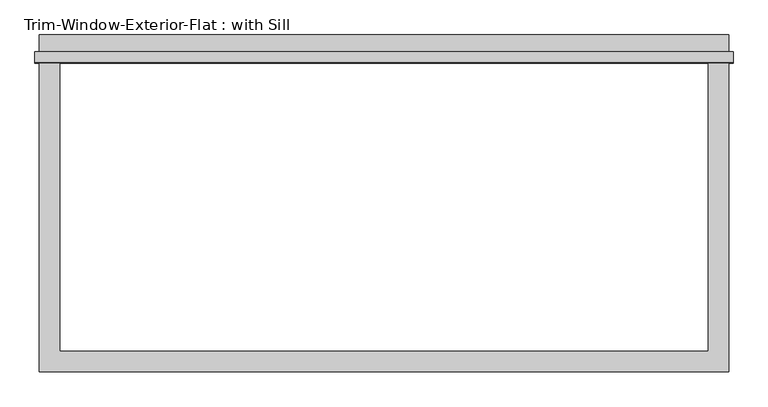
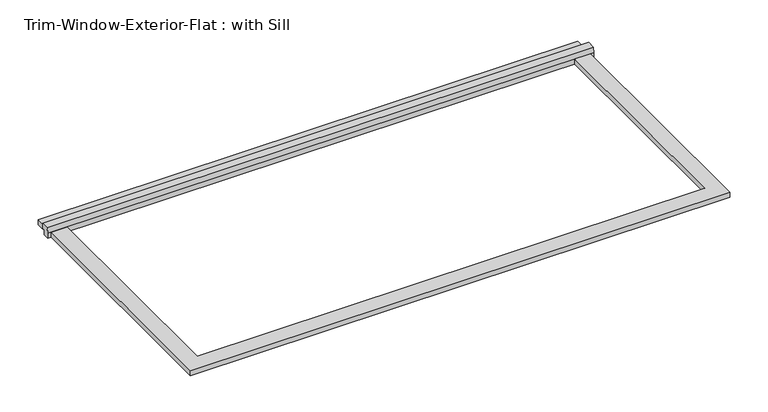
"""IFC4 building model written with IfcOpenShell, lengths in millimetres: proxy geometry, Trim-Window-Exterior-Flat : with Sill."""

from ifc_helpers import new_model, si_unit, frame, origin, origin_with_axes, place, context, project, spatial, polyline, outline, extrude, source, transform, mapped, element, save


def trim_window_exterior_flat_with_sill_7b949e88(model_context):
    return source(origin(), model_context, "Body", "SweptSolid", [
        extrude(outline(polyline([(971.55, 834.9823709), (-971.55, 834.9823709), (-971.55, 892.1323709), (971.55, 892.1323709), (971.55, 834.9823709)])), origin_with_axes(), (0.0, 0.0, 1.0), 19.05),
        extrude(outline(polyline([(844.55, 38.1), (844.55, 19.05), (834.9823709, 19.05), (834.9823709, 0.0), (812.8, 0.0), (812.8, 19.05), (815.2580645, 38.1), (844.55, 38.1)])), frame((-984.25, 0.0, 0.0), z_axis=(1.0, 0.0, 0.0), x_axis=(0.0, 1.0, 0.0)), (0.0, 0.0, 1.0), 1968.5),
        extrude(outline(polyline([(-971.55, -57.15), (-971.55, 812.8), (-914.4, 812.8), (-914.4, 0.0), (914.4, 0.0), (914.4, 812.8), (971.55, 812.8), (971.55, -57.15), (-971.55, -57.15)])), origin_with_axes(), (0.0, 0.0, 1.0), 19.05),
    ])


if __name__ == "__main__":
    model = new_model("IFC4")
    model_context = context("Model", 3, world=origin())
    ifc_project = project(units=[si_unit("LENGTHUNIT", "METRE", prefix="MILLI")], contexts=[model_context])
    site = spatial("IfcSite", under=ifc_project)
    building = spatial("IfcBuilding", under=site)
    placement = place(None, origin())
    trim_window_exterior_flat_with_sill_shape = trim_window_exterior_flat_with_sill_7b949e88(model_context)
    element("IfcBuildingElementProxy", 1, Name="Trim-Window-Exterior-Flat : with Sill", ObjectType="Trim-Window-Exterior-Flat : with Sill", at=placement, inside=building, context=model_context, shape_type="MappedRepresentation", body=[
        mapped(trim_window_exterior_flat_with_sill_shape, transform((0.0, 0.0, 0.0), x_axis=(1.0, 0.0, 0.0), y_axis=(0.0, 1.0, 0.0), z_axis=(0.0, 0.0, 1.0))),
    ])
    save(model, "model.ifc")

# Revit data of these elements
# Type "Trim-Window-Exterior-Flat : with Sill"
#   Trim Width = 0.1875 ft
#   Trim Thickness_Picture Frame = 0.104167 ft
#   Trim Thickness_with Sill = 0.0625 ft
#   Sill Thickness = 0.104167 ft
#   Opening Width [instance default] = 2 ft
#   Opening Height [instance default] = 3 ft
#   Default Elevation = 4 ft
#   Sill = yes
#   Picture Frame = no
#   Trim Material [instance default] = none
# Element 1 (IfcBuildingElementProxy, "Trim-Window-Exterior-Flat : with Sill")
#   Opening Width = 6 ft
#   Opening Height = 2.666667 ft
#   Trim Material = Clad - White
#   Materials on its faces: "Clad - White"
# Materials
#   "Clad - White": class "Wood", colour RGB 242 242 238, transparency 0, Cost = 0
